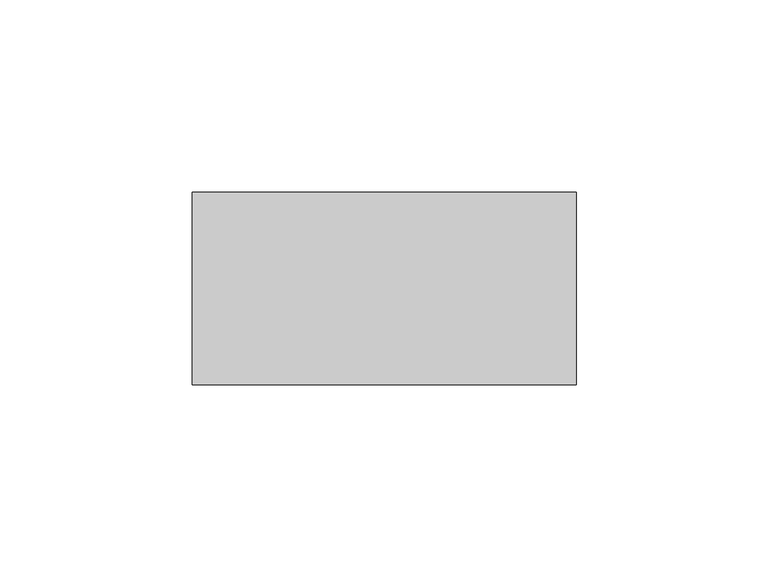
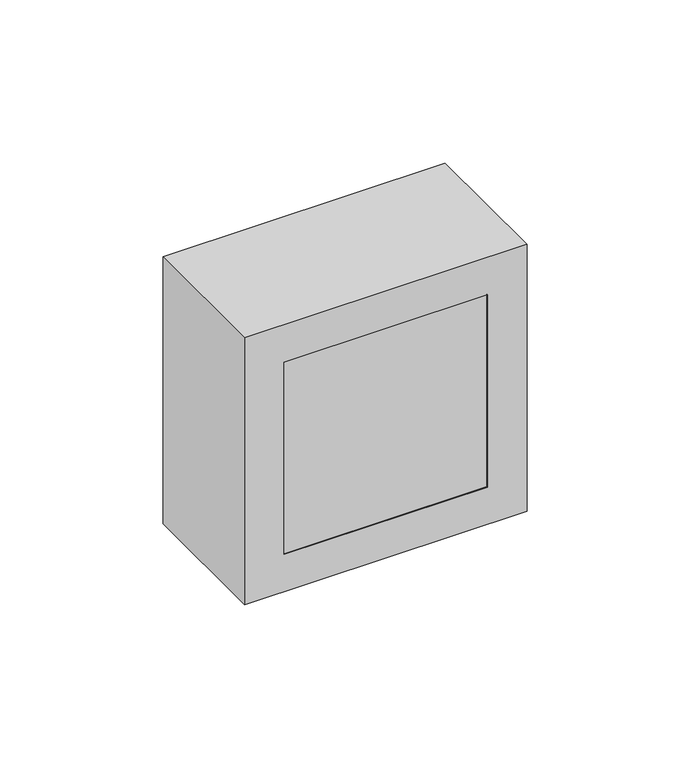
"""IFC4 building model written with IfcOpenShell, lengths in millimetres: light fixture geometry."""

from ifc_helpers import new_model, si_unit, frame, origin, place, context, project, spatial, polyline, outline, extrude, source, transform, mapped, element, save


def light_fixture_da35b629(model_context):
    return source(origin(), model_context, "Body", "SweptSolid", [
        extrude(outline(polyline([(1950.0, -86.3556627), (1950.0, 13.6443373), (2050.0, 13.6443373), (2050.0, -86.3556627), (1950.0, -86.3556627)]), holes=[polyline([(2036.0, -72.3556627), (2036.0, -0.3556627), (1964.0, -0.3556627), (1964.0, -72.3556627), (2036.0, -72.3556627)])]), frame((0.0, 45.1, 0.0), z_axis=(0.0, 1.0, 0.0), x_axis=(0.0, 0.0, 1.0)), (0.0, 0.0, 1.0), 50.2),
        extrude(outline(polyline([(-0.3556627, 45.1), (-72.3556627, 45.1), (-72.3556627, 66.0166667), (-0.3556627, 66.0166667), (-0.3556627, 45.1)])), frame((0.0, 0.0, 1964.0), z_axis=(0.0, 0.0, 1.0), x_axis=(1.0, 0.0, 0.0)), (0.0, 0.0, 1.0), 72.0),
    ])


if __name__ == "__main__":
    model = new_model("IFC4")
    model_context = context("Model", 3, world=origin())
    ifc_project = project(units=[si_unit("LENGTHUNIT", "METRE", prefix="MILLI")], contexts=[model_context])
    site = spatial("IfcSite", under=ifc_project)
    building = spatial("IfcBuilding", under=site)
    placement = place(None, origin())
    light_fixture_shape = light_fixture_da35b629(model_context)
    element("IfcLightFixture", 1, at=placement, inside=building, context=model_context, shape_type="MappedRepresentation", body=[
        mapped(light_fixture_shape, transform((0.0, 0.0, 0.0), x_axis=(1.0, 0.0, 0.0), y_axis=(0.0, 1.0, 0.0), z_axis=(0.0, 0.0, 1.0))),
    ])
    save(model, "model.ifc")

# Revit data of these elements
# Type
#   rahmen dicke = 0' - 0.98819"
#   rahmen breite(okvir) = 0' - 0.55118"
#   rahmen breite = 0' - 1.9685"
#   glas dicke = 0' - 0.82349"
#   abstand von wand (lichtquelle) = 0' - 2.76378"
#   Wattage = 20.16 W
#   Emit from Circle Diameter = 0' - 4.31496"
#   built-in parameter 1150110 = 1 (stored number, unit not read)
#   built-in parameter 1114217 = 1 (stored number, unit not read)
#   built-in parameter 1150109 = 1 (stored number, unit not read)
#   built-in parameter 1150113 = 1 (stored number, unit not read)
#   Lumens = 2994.61 lm
#   built-in parameter 1150115 = 1 (stored number, unit not read)
#   built-in parameter 1150105 = 953.213 (stored number, unit not read)
#   Light Source Symbol Size = 2' - 0"
#   built-in parameter 1150112 = 1 (stored number, unit not read)
#   built-in parameter 1150114 = 1 (stored number, unit not read)
#   built-in parameter 1150107 = 3000 (stored number, unit not read)
#   built-in parameter 1150106 = 9.53213 (stored number, unit not read)
#   built-in parameter 1150104 = 13.8 (stored number, unit not read)
#   built-in parameter 1114218 = 1 (stored number, unit not read)
#   built-in parameter 1150133 = 10 (stored number, unit not read)
#   Emit Shape Visible in Rendering = yes
#   Color Filter = 16744448
#   rahmen material = rahmen material
#   glass material = glas material
#   Dimming Lamp Color Temperature Shift = (empty or 0)
#   Default Elevation = 0
# Element 1 (IfcLightFixture)
#   Materials on its faces: "rahmen material", "glas material"
# Materials
#   "rahmen material": class "Glas", colour RGB 0 0 255, transparency 0.75
#   "glas material": class "Glas", colour RGB 0 128 192, transparency 0.9
